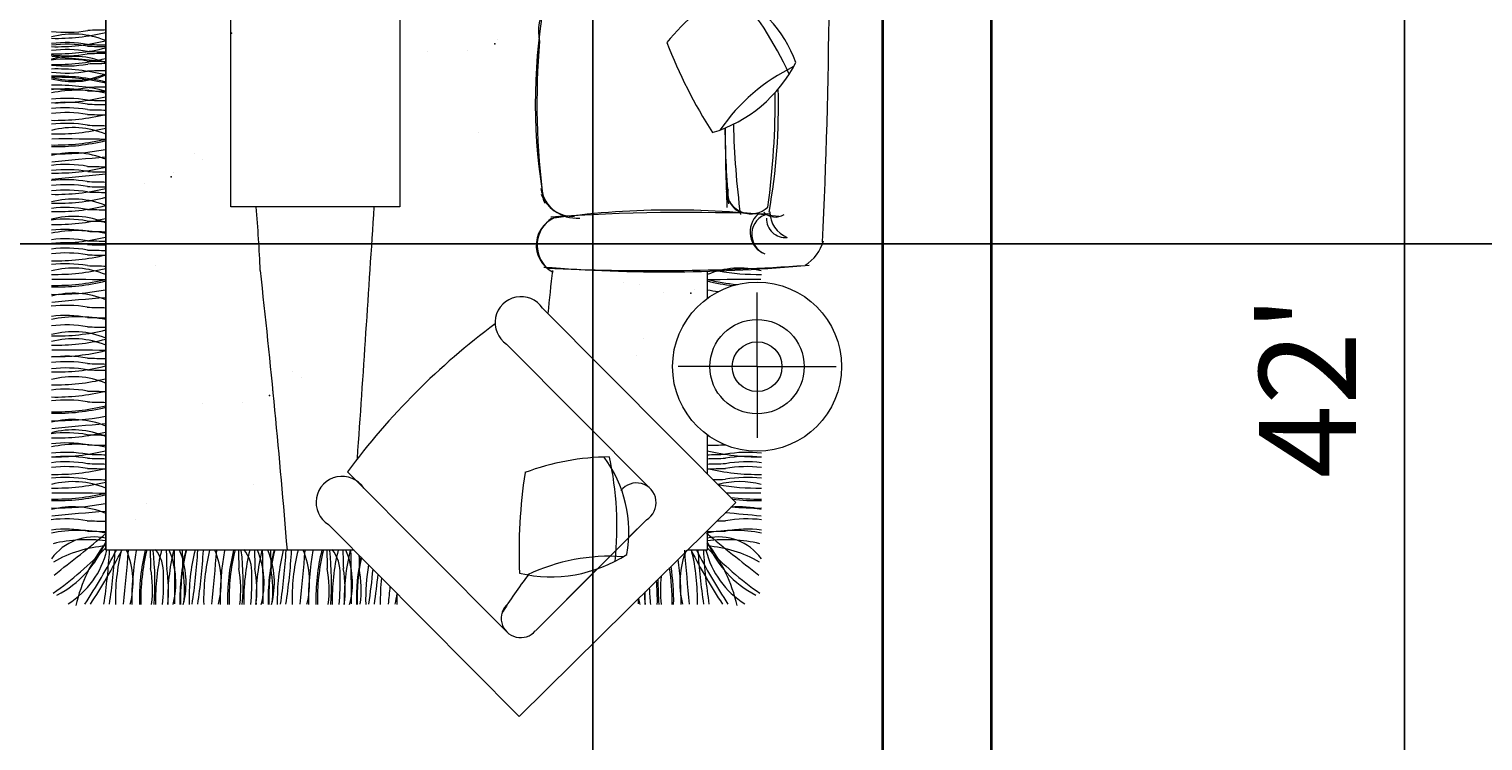
# Model space of a CAD drawing. Units: inches. Extents: x 502 to 1235, y -850 to 110.
# Tile 6 of 9: x 931 to 1051, y -335 to -277. Entities that reach past the tile are written whole.
import ezdxf

# ---------------------------------------------------------------- set-up
doc = ezdxf.new("R2010")
doc.units = ezdxf.units.IN
doc.header["$MEASUREMENT"] = 0
doc.layers.add('A-ANNO-DIMS', color=2, linetype='Continuous', lineweight=18)
doc.layers.add('WALL', color=1, linetype='Continuous', lineweight=35)
doc.layers.add('furniture', color=50, linetype='Continuous', lineweight=13, transparency=0.8)
doc.styles.get("Standard").update_dxf_attribs({"font": 'arial.ttf'})
doc.dimstyles.get("Standard").update_dxf_attribs({"dimtxt": 0.18, "dimasz": 0.18, "dimexe": 0.18, "dimexo": 0.0625, "dimgap": 0.09, "dimtad": 0, "dimtih": 1, "dimtoh": 1, "dimdec": 1, "dimzin": 0, "dimdsep": 46, "dimlunit": 4, "dimtxsty": 'Standard', "dimcen": 0.09, "dimadec": 0, "dimazin": 0, "dimtfac": 1, "dimtdec": 1, "dimtofl": 0, "dimtmove": 0, "dimatfit": 3, "dimfxl": 1, "dimtolj": 1, "dimtzin": 0, "dimarcsym": 0})

# ---------------------------------------------------------------- blocks, each defined once
blk = doc.blocks.new('_ArchTick')
at = {"color": 0, "linetype": 'ByBlock', "const_width": 0.15}
blk.add_lwpolyline([(-0.5, -0.5), (0.5, 0.5)], dxfattribs=at)
blk = doc.blocks.new('*D7')
at = {"layer": 'A-ANNO-DIMS', "color": 0, "lineweight": -2, "transparency": 16777216}
for p, q in [((1043.54, -60.85), (1044.72, -60.85)), ((1044.54, -60.85), (1044.54, -551.48)), ((1043.54, -551.48), (1044.72, -551.48))]:
    blk.add_line(p, q, dxfattribs=at)
at = {"layer": 'Defpoints', "color": 0, "transparency": 16777216}
for p in [(1010.39, -60.85), (1010.39, -551.48), (1044.54, -551.48)]:
    blk.add_point(p, dxfattribs=at)
at = {"layer": 'A-ANNO-DIMS', "color": 0, "lineweight": -2, "transparency": 16777216, "xscale": 5, "yscale": 5, "zscale": 5}
for p, rotation in [((1044.54, -60.85), 90), ((1044.54, -551.48), 270)]:
    blk.add_blockref('_ArchTick', p, dxfattribs=dict(at, rotation=rotation))
at = {"layer": 'A-ANNO-DIMS', "color": 0, "transparency": 16777216, "insert": (1036.52, -306.16), "char_height": 8, "attachment_point": 5, "rotation": 90}
blk.add_mtext("\\A1;42'", dxfattribs=at)
blk = doc.blocks.new('*D28')
at = {"layer": 'A-ANNO-DIMS', "color": 0, "lineweight": -2, "transparency": 16777216}
for p, q in [((770.85, -217.85), (1235.01, -217.85)), ((1234.83, -218.03), (1234.83, -255.91)), ((1234.83, -294.17), (1234.83, -256.28)), ((770.85, -294.35), (1235.01, -294.35))]:
    blk.add_line(p, q, dxfattribs=at)
at = {"layer": 'A-ANNO-DIMS', "color": 0, "transparency": 16777216}
for points in [[(1234.8, -218.03), (1234.86, -218.03), (1234.83, -217.85)], [(1234.8, -294.17), (1234.86, -294.17), (1234.83, -294.35)]]:
    blk.add_solid(points, dxfattribs=at)
at = {"layer": 'Defpoints', "color": 0, "transparency": 16777216}
for p in [(770.79, -217.85), (770.79, -294.35), (1234.83, -294.35)]:
    blk.add_point(p, dxfattribs=at)
at = {"layer": 'A-ANNO-DIMS', "color": 0, "transparency": 16777216, "insert": (1234.83, -256.1), "char_height": 0.18, "attachment_point": 5}
blk.add_mtext('\\A1;6\'-4 1/2"', dxfattribs=at)
blk = doc.blocks.new('*D43')
at = {"layer": 'A-ANNO-DIMS', "color": 0, "lineweight": -2, "transparency": 16777216}
for p, q in [((977.39, -422.28), (977.39, 63.98)), ((977.57, 63.8), (989.06, 63.8)), ((1001.21, 63.8), (989.72, 63.8)), ((1001.39, -422.28), (1001.39, 63.98))]:
    blk.add_line(p, q, dxfattribs=at)
at = {"layer": 'A-ANNO-DIMS', "color": 0, "transparency": 16777216}
for points in [[(977.57, 63.83), (977.57, 63.77), (977.39, 63.8)], [(1001.21, 63.83), (1001.21, 63.77), (1001.39, 63.8)]]:
    blk.add_solid(points, dxfattribs=at)
at = {"layer": 'Defpoints', "color": 0, "transparency": 16777216}
for p in [(1001.39, 63.8), (977.39, -422.35), (1001.39, -422.35)]:
    blk.add_point(p, dxfattribs=at)
at = {"layer": 'A-ANNO-DIMS', "color": 0, "transparency": 16777216, "insert": (989.39, 63.8), "char_height": 0.18, "attachment_point": 5}
blk.add_mtext('\\A1;2\'-0"', dxfattribs=at)

msp = doc.modelspace()

# ---------------------------------------------------------------- linework, layer by layer
at = {"layer": 'furniture'}
for p, q in [((937.11, -319.68), (937.11, -230.81)), ((937.11, -244.85), (937.11, -319.68)), ((947.46, -291.3), (947.46, -257.76)), ((961.43, -257.76), (961.43, -291.3)), ((969.51, -277.43), (969.51, -277.43)), ((935.71, -278.42), (935.71, -278.42)), ((963.76, -278.44), (963.76, -278.44)), ((967.07, -278.39), (967.07, -278.39)), ((935.71, -281.45), (935.71, -281.45)), ((935.71, -281.55), (935.71, -281.55)), ((967.96, -285.13), (967.96, -285.13)), ((944.42, -286.86), (944.42, -286.86)), ((944.42, -286.86), (944.42, -286.86)), ((945.15, -287.34), (945.15, -287.34)), ((945.15, -287.34), (945.15, -287.34)), ((942.75, -288.42), (942.75, -288.42)), ((937, -289.44), (937, -289.44)), ((940.31, -289.39), (940.31, -289.39)), ((961.43, -291.3), (947.46, -291.3)), ((941.2, -296.12), (941.2, -296.12)), ((986.86, -296.62), (986.86, -298.87)), ((979.93, -297.59), (979.93, -297.59)), ((981.28, -297.7), (981.28, -297.7)), ((985.82, -298.13), (985.82, -298.13)), ((983.21, -298.38), (983.21, -298.38)), ((990.99, -304.51), (990.99, -298.39)), ((989.22, -315.75), (973.24, -299.68)), ((982.16, -314.61), (970.27, -302.64)), ((981.63, -302.22), (981.63, -302.22)), ((980.99, -303.55), (980.99, -303.55)), ((952.55, -304.95), (952.55, -304.95)), ((952.55, -304.95), (952.55, -304.95)), ((953.28, -305.44), (953.28, -305.44)), ((953.28, -305.44), (953.28, -305.44)), ((990.99, -304.51), (984.45, -304.51)), ((990.99, -304.51), (990.99, -310.4)), ((990.99, -304.51), (997.54, -304.51)), ((950.88, -306.52), (950.88, -306.52)), ((945.13, -307.53), (945.13, -307.53)), ((948.44, -307.48), (948.44, -307.48)), ((986.86, -310.14), (986.86, -313.38)), ((957.1, -313.2), (970.29, -326.45)), ((949.33, -314.22), (949.33, -314.22)), ((940.49, -315.83), (940.49, -315.83)), ((989.22, -315.75), (971.31, -333.43)), ((935.97, -317.19), (935.97, -317.19)), ((935.97, -317.19), (935.97, -317.19)), ((935.97, -317.19), (935.97, -317.19)), ((939.54, -317.17), (939.54, -317.17)), ((981.84, -317.17), (972.65, -326.35)), ((981.84, -317.17), (980.36, -318.64)), ((988, -317.19), (988, -317.19)), ((988, -317.19), (988, -317.19)), ((988, -317.19), (988, -317.19)), ((935.71, -318.27), (935.71, -318.27)), ((935.71, -318.27), (935.71, -318.27)), ((935.71, -318.27), (935.71, -318.27)), ((971.31, -333.43), (955.54, -317.56)), ((986.86, -318.07), (986.86, -319.68)), ((988.26, -318.27), (988.26, -318.27)), ((988.26, -318.27), (988.26, -318.27)), ((988.26, -318.27), (988.26, -318.27)), ((957.65, -319.68), (937.11, -319.68)), ((986.86, -319.68), (985.23, -319.68)), ((943.83, -322.07), (943.83, -322.07)), ((951.13, -322.07), (951.13, -322.07)), ((958.44, -322.07), (958.44, -322.07)), ((977.77, -321.23), (972.65, -326.35)), ((943.79, -322.49), (943.79, -322.49)), ((951.09, -322.49), (951.09, -322.49)), ((958.4, -322.49), (958.4, -322.49))]:
    msp.add_line(p, q, dxfattribs=at)
for radius in [6.99, 3.9, 2.06]:
    msp.add_circle((990.99, -304.51), radius, dxfattribs=at)
for centre, radius, start, end in [((497.35, -270.42), 499.62, 357.2697, 1.7875), ((976.54, -276.76), 3.64, 96.5867, 193.4511), ((999.11, -290.54), 20.19, 120.3068, 140.5663), ((984.48, -282.8), 10.3, 19.4501, 66.7699), ((968.74, -291.45), 27.27, 24.0815, 42.2768), ((1018.67, -282.68), 46.03, 170.0543, 190.4167), ((933.02, -261.02), 17.03, 268.6331, 283.8573), ((933.04, -260.33), 17.03, 268.6331, 283.8573), ((934.42, -283.99), 6.98, 67.3098, 104.8613), ((933.84, -287.82), 10.11, 79.9349, 96.8829), ((933.85, -266.75), 10.11, 263.1171, 280.0651), ((939.18, -389.41), 112.76, 91.0225, 91.8109), ((1034.24, -282.74), 61.46, 175.2072, 187.551), ((1023.76, -261.99), 43.2, 201.3371, 212.4176), ((933.82, -268.69), 10.11, 263.1171, 280.0651), ((934.41, -285.83), 6.98, 67.3098, 104.8613), ((933.84, -287.96), 10.11, 79.9349, 96.8829), ((933.04, -261.61), 17.03, 268.6331, 283.8573), ((933.84, -288.4), 10.11, 79.9349, 96.8829), ((897.72, -655.28), 378.04, 84.0165, 84.6992), ((939.15, -391.35), 112.76, 91.0225, 91.8109), ((939.17, -165.16), 112.76, 268.1891, 268.9775), ((939.17, -165.3), 112.76, 268.1891, 268.9775), ((939.17, -165.74), 112.76, 268.1891, 268.9775), ((933.02, -262.49), 17.03, 268.6331, 283.8573), ((933.82, -289.19), 10.11, 79.9349, 96.8829), ((933.02, -296.92), 17.03, 76.1427, 91.3669), ((933.84, -270.12), 10.11, 263.1171, 280.0651), ((933.85, -269.53), 10.11, 263.1171, 280.0651), ((939.15, -166.53), 112.76, 268.1891, 268.9775), ((939.17, -392.78), 112.76, 91.0225, 91.8109), ((939.18, -392.19), 112.76, 91.0225, 91.8109), ((983.91, -274.12), 11.54, 287.0126, 332.9429), ((1000.83, -293.75), 15.62, 115.9005, 145.6513), ((934.42, -273.85), 6.98, 255.1387, 292.6902), ((934.42, -273.95), 6.98, 255.1387, 292.6902), ((933.04, -297.51), 17.03, 76.1427, 91.3669), ((933.04, -297.61), 17.03, 76.1427, 91.3669), ((933.04, -298.26), 17.03, 76.1427, 91.3669), ((939.17, -394.13), 112.76, 91.0225, 91.8109), ((933.83, -291.65), 10.11, 79.9349, 96.8829), ((934.83, -292.97), 11.32, 78.4112, 101.2455), ((933.02, -265.65), 17.03, 268.6331, 283.8573), ((933.83, -292.43), 10.11, 79.9349, 96.8829), ((933.84, -271.47), 10.11, 263.1171, 280.0651), ((939.16, -168.99), 112.76, 268.1891, 268.9775), ((939.16, -169.77), 112.76, 268.1891, 268.9775), ((927.74, -282.47), 64.75, 352.1551, 0.5585), ((942.43, -282.94), 50.33, 349.9466, 1.5903), ((933.83, -292.76), 10.11, 79.9349, 96.8829), ((933.83, -293.21), 10.11, 79.9349, 96.8829), ((933.83, -293.61), 10.11, 79.9349, 96.8829), ((933.03, -267.11), 17.03, 268.6331, 283.8573), ((939.16, -170.1), 112.76, 268.1891, 268.9775), ((939.16, -170.55), 112.76, 268.1891, 268.9775), ((939.16, -170.95), 112.76, 268.1891, 268.9775), ((933.83, -294.5), 10.11, 79.9349, 96.8829), ((933.03, -268.24), 17.03, 268.6331, 283.8573), ((934.42, -291.72), 6.98, 67.3098, 104.8613), ((939.16, -171.84), 112.76, 268.1891, 268.9775), ((1085.26, -283.52), 96.94, 180.7456, 184.456), ((1108.91, -285.53), 120.55, 179.6386, 182.7653), ((1059.84, -282.76), 70.83, 181.3731, 187.4472), ((933.03, -269.15), 17.03, 268.6331, 283.8573), ((933.03, -269.28), 17.03, 268.6331, 283.8573), ((933.66, -431.48), 145.8, 88.628, 90.3934), ((933.01, -264.31), 22.61, 269.0195, 280.4039), ((934.42, -293.8), 6.98, 67.3098, 104.8613), ((952.74, -485.37), 198.79, 94.5146, 95.8017), ((933.84, -297.9), 10.11, 79.9349, 96.8829), ((933.04, -271.47), 17.03, 268.6331, 283.8573), ((933.85, -298.33), 10.11, 79.9349, 96.8829), ((897.72, 87.43), 378.04, 275.3008, 275.9835), ((939.17, -175.24), 112.76, 268.1891, 268.9775), ((939.18, -175.67), 112.76, 268.1891, 268.9775), ((933.82, -299.16), 10.11, 79.9349, 96.8829), ((933.84, -299.57), 10.11, 79.9349, 96.8829), ((933.04, -273.23), 17.03, 268.6331, 283.8573), ((939.15, -176.5), 112.76, 268.1891, 268.9775), ((939.17, -176.91), 112.76, 268.1891, 268.9775), ((976.06, -289.21), 3.02, 190.9756, 274.9747), ((933.84, -300.02), 10.11, 79.9349, 96.8829), ((933.04, -273.97), 17.03, 268.6331, 283.8573), ((934.42, -297.63), 6.98, 67.3098, 104.8613), ((939.17, -177.36), 112.76, 268.1891, 268.9775), ((975.77, -289.29), 2.8, 199.8228, 272.4985), ((990.48, -289.81), 2.06, 186.1174, 313.1189), ((990.2, -290.2), 1.63, 167.6226, 260.3094), ((933.02, -274.66), 17.03, 268.6331, 283.8573), ((934.41, -299.06), 6.98, 67.3098, 104.8613), ((933.84, -301.46), 10.11, 79.9349, 96.8829), ((939.17, -178.8), 112.76, 268.1891, 268.9775), ((771.24, -305.27), 178.87, 2.7877, 4.4807), ((-3027.9, -35.6), 3995.41, 356.03178, 356.33069), ((975.19, -294.47), 2.47, 104.6379, 244.3095), ((985.07, -453.3), 161.54, 87.5073, 93.9592), ((984.01, -363.63), 72.07, 82.9836, 97.989), ((992.38, -293.37), 1.97, 132.3134, 247.6102), ((992.3, -293.57), 1.75, 104.7814, 247.5922), ((992.49, -290.82), 1.32, 224.3938, 303.5856), ((993.31, -292.28), 1.55, 178.0108, 276.5585), ((994.37, -291.65), 2.34, 181.184, 247.8216), ((933.02, -275.72), 17.03, 268.6331, 283.8573), ((933.82, -302.42), 10.11, 79.9349, 96.8829), ((933.83, -303.27), 10.11, 79.9349, 96.8829), ((934.83, -304.58), 11.32, 78.4112, 101.2455), ((939.15, -179.76), 112.76, 268.1891, 268.9775), ((939.16, -180.61), 112.76, 268.1891, 268.9775), ((975.43, -294.46), 2.63, 123.041, 226.0653), ((933.02, -277.26), 17.03, 268.6331, 283.8573), ((933.83, -304.05), 10.11, 79.9349, 96.8829), ((933.83, -304.37), 10.11, 79.9349, 96.8829), ((939.16, -181.39), 112.76, 268.1891, 268.9775), ((939.16, -181.71), 112.76, 268.1891, 268.9775), ((993.09, -293.13), 3.53, 301.8817, 343.9672), ((933.83, -304.82), 10.11, 79.9349, 96.8829), ((933.83, -305.22), 10.11, 79.9349, 96.8829), ((933.03, -278.73), 17.03, 268.6331, 283.8573), ((939.16, -182.16), 112.76, 268.1891, 268.9775), ((939.16, -182.56), 112.76, 268.1891, 268.9775), ((933.83, -306.11), 10.11, 79.9349, 96.8829), ((933.03, -279.85), 17.03, 268.6331, 283.8573), ((934.42, -303.34), 6.98, 67.3098, 104.8613), ((939.16, -183.45), 112.76, 268.1891, 268.9775), ((129.64, -387.28), 825.27, 4.69873, 6.31076), ((983.38, -170.66), 126.01, 265.4325, 275.431), ((982.27, -111.62), 184.95, 267.3143, 273.933), ((1794.33, -387.28), 825.27, 173.68924, 173.93736), ((989.55, -303.34), 6.98, 75.1387, 112.6902), ((990.94, -279.85), 17.03, 259.3731, 271.3669), ((933.01, -275.92), 22.61, 269.0195, 280.4039), ((933.03, -280.76), 17.03, 268.6331, 283.8573), ((933.03, -280.89), 17.03, 268.6331, 283.8573), ((933.66, -443.1), 145.8, 88.628, 90.3934), ((990.31, -443.1), 145.8, 89.6066, 91.372), ((990.94, -280.76), 17.03, 256.1427, 264.5854), ((990.94, -280.89), 17.03, 256.1427, 263.4467), ((990.96, -275.92), 22.61, 259.5961, 261.862), ((933.82, -309.55), 10.11, 79.9349, 96.8829), ((934.42, -305.42), 6.98, 67.3098, 104.8613), ((952.74, -496.98), 198.79, 94.5146, 95.8017), ((971.46, -300.86), 2.14, 33.6335, 236.3665), ((933.83, -310.39), 10.11, 79.9349, 96.8829), ((934.83, -311.71), 11.32, 78.4112, 101.2455), ((939.15, -186.89), 112.76, 268.1891, 268.9775), ((939.16, -187.73), 112.76, 268.1891, 268.9775), ((933.83, -311.17), 10.11, 79.9349, 96.8829), ((933.04, -284.94), 17.03, 268.6331, 283.8573), ((934.42, -308.6), 6.98, 67.3098, 104.8613), ((939.16, -188.51), 112.76, 268.1891, 268.9775), ((1004.81, -348.64), 59.43, 126.6613, 143.3951), ((933.03, -285.7), 17.03, 268.6331, 283.8573), ((934.42, -309.18), 6.98, 67.3098, 104.8613), ((933.02, -286.65), 17.03, 268.6331, 283.8573), ((933.83, -313.76), 10.11, 79.9349, 96.8829), ((933.83, -314.21), 10.11, 79.9349, 96.8829), ((933.66, -448.94), 145.8, 88.628, 90.3934), ((939.16, -191.1), 112.76, 268.1891, 268.9775), ((933.02, -287.92), 17.03, 268.6331, 283.8573), ((934.41, -312.32), 6.98, 67.3098, 104.8613), ((933.84, -314.73), 10.11, 79.9349, 96.8829), ((939.16, -191.55), 112.76, 268.1891, 268.9775), ((939.17, -192.07), 112.76, 268.1891, 268.9775), ((933.02, -288.98), 17.03, 268.6331, 283.8573), ((933.83, -316.48), 10.11, 79.9349, 96.8829), ((933.03, -289.99), 17.03, 268.6331, 283.8573), ((939.16, -193.82), 112.76, 268.1891, 268.9775), ((933.83, -317.38), 10.11, 79.9349, 96.8829), ((933.03, -291.21), 17.03, 268.6331, 283.8573), ((939.16, -194.72), 112.76, 268.1891, 268.9775), ((933.01, -286.37), 22.61, 269.0195, 280.4039), ((933.03, -291.33), 17.03, 268.6331, 283.8573), ((934.42, -315.86), 6.98, 67.3098, 104.8613), ((933.02, -293.38), 17.03, 268.6331, 283.8573), ((933.82, -320.09), 10.11, 79.9349, 96.8829), ((934.41, -316.72), 6.98, 67.3098, 104.8613), ((952.74, -507.42), 198.79, 94.5146, 95.8017), ((939.15, -197.43), 112.76, 268.1891, 268.9775), ((984.82, -197.43), 112.76, 271.0225, 271.0606), ((989.56, -316.72), 6.98, 111.652, 112.6902), ((933.83, -320.93), 10.11, 79.9349, 96.8829), ((934.83, -322.25), 11.32, 78.4112, 101.2455), ((933.02, -294.93), 17.03, 268.6331, 283.8573), ((939.16, -198.27), 112.76, 268.1891, 268.9775), ((984.81, -198.27), 112.76, 271.0225, 271.8109), ((990.95, -294.93), 17.03, 256.1427, 271.3669), ((933.83, -321.71), 10.11, 79.9349, 96.8829), ((933.83, -322.04), 10.11, 79.9349, 96.8829), ((933.83, -322.49), 10.11, 79.9349, 96.8829), ((939.16, -199.05), 112.76, 268.1891, 268.9775), ((939.16, -199.38), 112.76, 268.1891, 268.9775), ((939.16, -199.82), 112.76, 268.1891, 268.9775), ((978.88, -332.17), 20.19, 90.3068, 110.5663), ((970.08, -318.15), 10.3, 349.4501, 36.7699), ((952.13, -317.78), 27.27, 354.0815, 12.2768), ((984.81, -199.05), 112.76, 271.0225, 271.8109), ((984.81, -199.38), 112.76, 271.0225, 271.8109), ((984.81, -199.82), 112.76, 271.0225, 271.8109), ((990.14, -322.04), 10.11, 83.1171, 100.0651), ((990.14, -322.49), 10.11, 83.1171, 100.0651), ((990.14, -321.71), 10.11, 83.1171, 100.0651), ((933.83, -322.89), 10.11, 79.9349, 96.8829), ((933.03, -296.39), 17.03, 268.6331, 283.8573), ((933.83, -323.78), 10.11, 79.9349, 96.8829), ((939.16, -200.22), 112.76, 268.1891, 268.9775), ((939.16, -201.12), 112.76, 268.1891, 268.9775), ((956.66, -315.73), 2.15, 33.0924, 238.5307), ((1014.5, -319.77), 43.2, 171.3371, 182.4176), ((984.81, -200.22), 112.76, 271.0225, 271.8109), ((990.94, -296.39), 17.03, 256.1427, 271.3669), ((984.81, -201.12), 112.76, 271.2964, 271.8109), ((990.14, -322.89), 10.11, 83.1171, 100.0651), ((990.14, -323.78), 10.11, 83.1171, 100.0651), ((933.03, -297.52), 17.03, 268.6331, 283.8573), ((934.42, -321), 6.98, 67.3098, 104.8613), ((933.03, -298.43), 17.03, 268.6331, 283.8573), ((933.66, -460.76), 145.8, 88.628, 90.3934), ((981.01, -315.76), 1.63, 300.4819, 142.3252), ((990.94, -297.52), 17.03, 259.2534, 271.3669), ((989.55, -321), 6.98, 75.1387, 104.8341), ((990.31, -460.76), 145.8, 89.6066, 90.7304), ((933.01, -293.59), 22.61, 269.0195, 280.4039), ((933.03, -298.56), 17.03, 268.6331, 283.8573), ((934.42, -323.08), 6.98, 67.3098, 104.8613), ((990.94, -298.43), 17.03, 262.7707, 271.3669), ((989.55, -323.08), 6.98, 75.1387, 96.0041), ((990.96, -293.59), 22.61, 264.6488, 270.9805), ((990.94, -298.56), 17.03, 263.2584, 271.3669), ((933.82, -327.21), 10.11, 79.9349, 96.8829), ((952.74, -514.65), 198.79, 94.5146, 95.8017), ((939.15, -204.55), 112.76, 268.1891, 268.9775), ((984.82, -204.55), 112.76, 271.4616, 271.8109), ((971.23, -514.65), 198.79, 84.1983, 85.0575), ((990.15, -327.21), 10.11, 83.1171, 100.0651), ((933.83, -328.06), 10.11, 79.9349, 96.8829), ((934.83, -329.37), 11.32, 78.4112, 101.2455), ((936.15, -322.94), 4.35, 77.1946, 144.0943), ((848.78, -212.37), 137.94, 307.5441, 309.8432), ((939.16, -205.4), 112.76, 268.1891, 268.9775), ((1075.19, -212.37), 137.94, 230.1568, 232.4559), ((984.81, -205.4), 112.76, 271.0225, 271.8109), ((987.82, -322.94), 4.35, 35.9057, 102.8054), ((989.14, -329.37), 11.32, 78.7545, 101.5888), ((990.14, -328.06), 10.11, 83.1171, 100.0651), ((935.58, -331.1), 12.28, 82.8509, 103.2785), ((915.4, -298.73), 30.04, 305.3153, 316.284), ((937.87, -329.52), 10.21, 94.2757, 119.865), ((929.13, -315.76), 8.61, 297.3033, 337.8819), ((930.08, -317.91), 7.35, 302.2712, 346.0065), ((947.54, -327.24), 13.24, 141.9231, 167.0477), ((893.44, -296.72), 50.12, 326.8219, 332.7331), ((893.89, -296.73), 50.12, 326.8219, 332.7331), ((888.83, -316.85), 48.68, 351.3771, 356.6356), ((889.29, -316.86), 48.68, 351.3771, 356.6356), ((954.94, -323.77), 17.03, 166.1427, 181.3669), ((740.82, -304.05), 198.79, 354.1983, 355.4854), ((932.39, -322.37), 6.98, 345.1387, 22.6902), ((961.88, -323.79), 22.61, 169.5961, 180.9805), ((956.92, -323.76), 17.03, 166.1427, 181.3669), ((957.04, -323.76), 17.03, 166.1427, 181.3669), ((1053.53, -317.63), 112.76, 181.0225, 181.8109), ((918.17, -322.37), 23.01, 355.4936, 6.6298), ((938.84, -321.53), 3.05, 356.8256, 38.3436), ((958.26, -323.76), 17.03, 166.1427, 181.3669), ((1054.86, -317.63), 112.76, 181.0225, 181.8109), ((959.27, -323.77), 17.03, 166.1427, 181.3669), ((935.93, -322.39), 6.98, 345.1387, 22.6902), ((797.03, -323.13), 145.8, 359.6066, 1.372), ((936.78, -322.38), 6.98, 345.1387, 22.6902), ((960.27, -323.76), 17.03, 166.1427, 181.3669), ((960.32, -323.77), 17.03, 166.1427, 181.3669), ((1056.18, -317.62), 112.76, 181.0225, 181.8109), ((961.03, -323.76), 17.03, 166.1427, 181.3669), ((896.13, -316.85), 48.68, 351.3771, 356.6356), ((896.59, -316.86), 48.68, 351.3771, 356.6356), ((962.24, -323.77), 17.03, 166.1427, 181.3669), ((748.12, -304.05), 198.79, 354.1983, 355.4854), ((939.69, -322.37), 6.98, 345.1387, 22.6902), ((969.18, -323.79), 22.61, 169.5961, 180.9805), ((964.22, -323.76), 17.03, 166.1427, 181.3669), ((964.34, -323.76), 17.03, 166.1427, 181.3669), ((1060.83, -317.63), 112.76, 181.0225, 181.8109), ((925.47, -322.37), 23.01, 355.4936, 6.6298), ((946.15, -321.53), 3.05, 356.8256, 38.3436), ((965.56, -323.76), 17.03, 166.1427, 181.3669), ((1062.16, -317.63), 112.76, 181.0225, 181.8109), ((966.57, -323.77), 17.03, 166.1427, 181.3669), ((943.23, -322.39), 6.98, 345.1387, 22.6902), ((804.33, -323.13), 145.8, 359.6066, 1.372), ((944.08, -322.38), 6.98, 345.1387, 22.6902), ((967.57, -323.76), 17.03, 166.1427, 181.3669), ((967.62, -323.77), 17.03, 166.1427, 181.3669), ((1063.48, -317.62), 112.76, 181.0225, 181.8109), ((968.33, -323.76), 17.03, 166.1427, 181.3669), ((903.44, -316.85), 48.68, 351.3771, 356.6356), ((903.89, -316.86), 48.68, 351.3771, 356.6356), ((969.55, -323.77), 17.03, 166.1427, 181.3669), ((755.43, -304.05), 198.79, 354.1983, 355.4854), ((947, -322.37), 6.98, 345.1387, 22.6902), ((976.49, -323.79), 22.61, 169.5961, 180.9805), ((971.52, -323.76), 17.03, 166.1427, 181.3669), ((971.65, -323.76), 17.03, 166.1427, 181.3669), ((1068.14, -317.63), 112.76, 181.0225, 181.8109), ((932.78, -322.37), 23.01, 355.4936, 6.6298), ((953.45, -321.53), 3.05, 356.8256, 38.3436), ((972.87, -323.76), 17.03, 166.1427, 181.3669), ((1069.47, -317.63), 112.76, 181.0225, 181.8109), ((973.87, -323.77), 17.03, 166.1427, 181.3669), ((950.54, -322.39), 6.98, 345.1387, 22.6902), ((811.63, -323.13), 145.8, 359.6066, 1.372), ((991.58, -322.37), 6.98, 157.3098, 194.8613), ((1183.15, -304.05), 198.79, 184.5146, 185.8017), ((1030.08, -296.73), 50.12, 207.2669, 213.1781), ((969.03, -323.77), 17.03, 358.6331, 13.8573), ((1030.53, -296.72), 50.12, 207.2669, 213.1781), ((1034.69, -316.86), 48.68, 183.3644, 188.6229), ((1035.14, -316.85), 48.68, 183.3644, 188.6229), ((993.89, -317.91), 7.35, 193.9935, 237.7288), ((988.39, -331.1), 12.28, 76.7215, 97.1491), ((994.84, -315.76), 8.61, 202.1181, 242.6967), ((976.44, -327.24), 13.24, 12.9523, 38.0769), ((986.1, -329.52), 10.21, 60.135, 85.7243), ((1008.57, -298.73), 30.04, 223.716, 234.6847), ((974.88, -323.76), 17.03, 168.0993, 181.3669), ((974.93, -323.77), 17.03, 168.2362, 181.3669), ((1070.79, -317.62), 112.76, 181.2535, 181.8109), ((975.64, -323.76), 17.03, 170.3159, 181.3669), ((973.93, -310.35), 11.54, 257.0126, 302.9429), ((978.77, -335.81), 15.62, 85.9005, 115.6513), ((967.06, -323.76), 17.03, 358.6331, 9.2236), ((962.09, -323.79), 22.61, 359.0195, 8.4847), ((930.87, -322.96), 10.11, 353.1171, 10.0651), ((926.14, -322.41), 15.76, 353.5587, 2.5565), ((932.2, -322.96), 10.11, 353.1171, 10.0651), ((933.52, -322.95), 10.11, 353.1171, 10.0651), ((938.17, -322.96), 10.11, 353.1171, 10.0651), ((933.44, -322.41), 15.76, 353.5587, 2.5565), ((939.5, -322.96), 10.11, 353.1171, 10.0651), ((940.82, -322.95), 10.11, 353.1171, 10.0651), ((945.48, -322.96), 10.11, 353.1171, 10.0651), ((940.75, -322.41), 15.76, 353.5587, 2.5565), ((946.81, -322.96), 10.11, 353.1171, 10.0651), ((948.13, -322.95), 10.11, 353.1171, 10.0651), ((910.74, -316.85), 48.68, 351.3771, 354.7986), ((911.2, -316.86), 48.68, 351.3771, 354.3194), ((976.85, -323.77), 17.03, 173.9229, 181.3669), ((996.78, -341.15), 31.42, 141.8457, 148.9133), ((965.71, -323.76), 17.03, 358.6331, 5.2422), ((1005.8, -322.37), 23.01, 179.2987, 184.5064), ((993.1, -322.96), 10.11, 173.6069, 186.8829), ((966.93, -323.76), 17.03, 358.6331, 8.8561), ((762.73, -304.05), 198.79, 354.1983, 354.6171), ((954.3, -322.37), 6.98, 345.1387, 352.5478), ((983.79, -323.79), 22.61, 178.619, 180.9805), ((991.77, -322.96), 10.11, 181.3666, 186.8829), ((964.71, -323.77), 17.03, 358.6331, 2.1135), ((997.83, -322.41), 15.76, 181.4332, 186.4413), ((971.42, -325.32), 1.6, 130.1092, 319.8908), ((1126.95, -323.13), 145.8, 180.2284, 180.3934), ((988.04, -322.39), 6.98, 190.6792, 194.8613)]:
    msp.add_arc(centre, radius, start, end, dxfattribs=at)
for p in [(947.51, -276.93), (969.3, -277.81), (942.53, -288.81), (985.51, -298.44), (950.67, -306.9)]:
    msp.add_point(p, dxfattribs=at)
at = {"layer": 'WALL'}
for p, q in [((1010.39, -615.85), (1010.39, -60.85)), ((1001.39, -418.35), (1001.39, -193.85))]:
    msp.add_line(p, q, dxfattribs=at)

# ---------------------------------------------------------------- dimensions: what is measured, and where the dimension line sits
at = {"layer": 'A-ANNO-DIMS'}
dim = msp.add_linear_dim(base=(1001.39, 63.8), p1=(977.39, -422.35), p2=(1001.39, -422.35), dimstyle='Standard', override={"dimdec": 1, "dimlfac": 1, "dimrnd": 0, "dimzin": 1, "dimdsep": 46, "dimlunit": 4, "dimfrac": 2}, dxfattribs=at)
dim.commit()
dim.dimension.update_dxf_attribs({"geometry": '*D43', "text_midpoint": (989.39, 63.8)})
dim = msp.add_linear_dim(base=(1044.54, -551.48), p1=(1010.39, -60.85), p2=(1010.39, -551.48), angle=90, text="42'", dimstyle='Standard', override={"dimtxt": 8, "dimasz": 5, "dimgap": 4, "dimtad": 1, "dimtih": 0, "dimblk1": 'ArchTick', "dimblk2": 'ArchTick', "dimsah": 1, "dimclrd": 0, "dimclre": 0, "dimclrt": 0, "dimfxlon": 1}, dxfattribs=at)
dim.commit()
dim.dimension.update_dxf_attribs({"geometry": '*D7', "text_midpoint": (1036.52, -306.16)})
dim = msp.add_linear_dim(base=(1234.83, -294.35), p1=(770.79, -217.85), p2=(770.79, -294.35), angle=90, dimstyle='Standard', override={"dimdec": 1, "dimlfac": 1, "dimrnd": 0, "dimzin": 1, "dimdsep": 46, "dimlunit": 4, "dimfrac": 2}, dxfattribs=at)
dim.commit()
dim.dimension.update_dxf_attribs({"geometry": '*D28', "text_midpoint": (1234.83, -256.1)})

doc.saveas('drawing.dxf')
